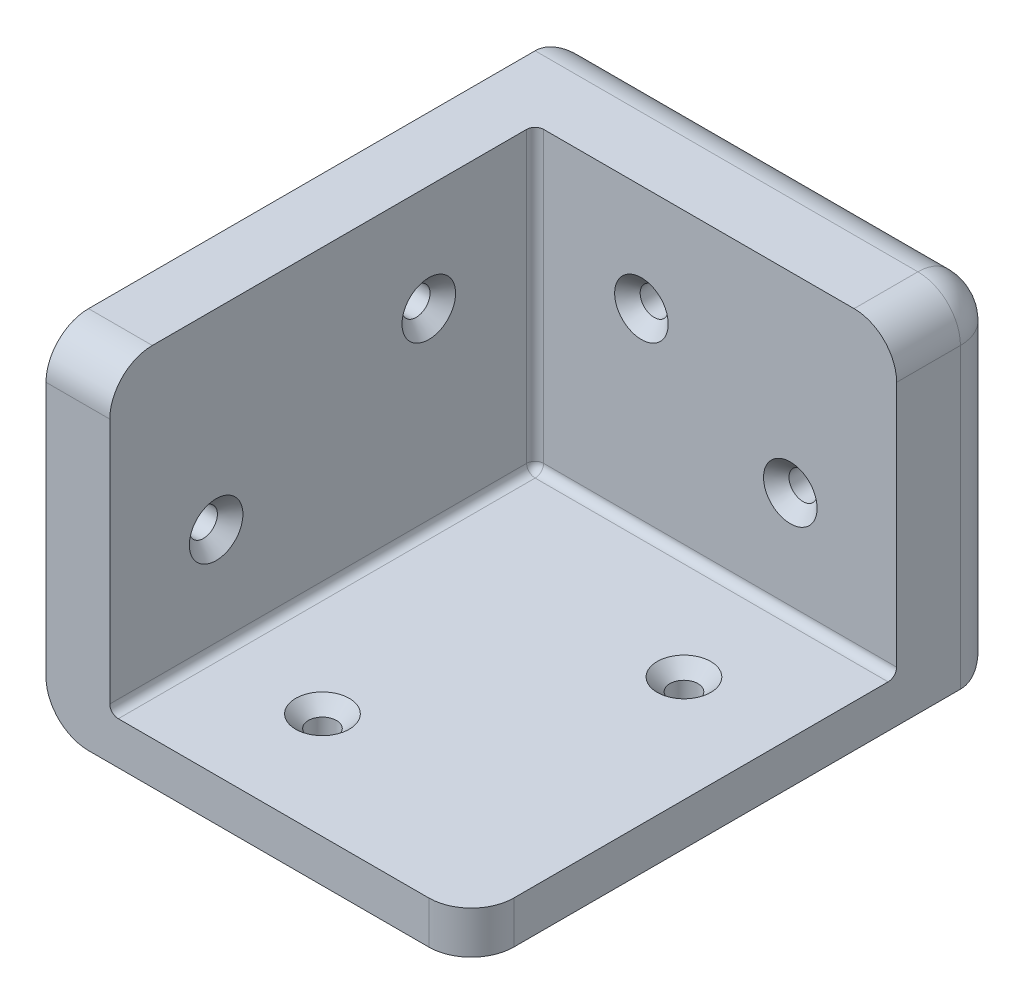
ISO-10303-21;
HEADER;
FILE_DESCRIPTION(('STEP AP214'),'2;1');
FILE_NAME('part.step','',(''),(''),'','','');
FILE_SCHEMA(('AUTOMOTIVE_DESIGN { 1 0 10303 214 1 1 1 1 }'));
ENDSEC;
DATA;
#1=APPLICATION_CONTEXT('core data for automotive mechanical design processes');
#2=APPLICATION_PROTOCOL_DEFINITION('international standard','automotive_design',2000,#1);
#3=PRODUCT_CONTEXT('',#1,'mechanical');
#4=PRODUCT('Part','Part','',(#3));
#5=PRODUCT_RELATED_PRODUCT_CATEGORY('part','',(#4));
#6=PRODUCT_DEFINITION_FORMATION('','',#4);
#7=PRODUCT_DEFINITION_CONTEXT('part definition',#1,'design');
#8=PRODUCT_DEFINITION('design','',#6,#7);
#9=PRODUCT_DEFINITION_SHAPE('','',#8);
#10=(LENGTH_UNIT() NAMED_UNIT(*) SI_UNIT(.MILLI.,.METRE.));
#11=(NAMED_UNIT(*) PLANE_ANGLE_UNIT() SI_UNIT($,.RADIAN.));
#12=(NAMED_UNIT(*) SI_UNIT($,.STERADIAN.) SOLID_ANGLE_UNIT());
#13=UNCERTAINTY_MEASURE_WITH_UNIT(LENGTH_MEASURE(1.E-05),#10,'distance_accuracy_value','');
#14=(GEOMETRIC_REPRESENTATION_CONTEXT(3) GLOBAL_UNCERTAINTY_ASSIGNED_CONTEXT((#13)) GLOBAL_UNIT_ASSIGNED_CONTEXT((#10,
#11,#12)) REPRESENTATION_CONTEXT('',''));
#15=CARTESIAN_POINT('',(0.,0.,0.));
#16=DIRECTION('',(0.,0.,1.));
#17=DIRECTION('',(1.,0.,0.));
#18=AXIS2_PLACEMENT_3D('',#15,#16,#17);
#19=CARTESIAN_POINT('',(-50.,40.,125.));
#20=DIRECTION('',(1.,0.,0.));
#21=DIRECTION('',(0.,1.,0.));
#22=AXIS2_PLACEMENT_3D('',#19,#20,#21);
#23=PLANE('',#22);
#24=CARTESIAN_POINT('',(-50.,-5.00000000000002,100.));
#25=DIRECTION('',(1.,0.,0.));
#26=DIRECTION('',(0.,1.,0.));
#27=AXIS2_PLACEMENT_3D('',#24,#25,#26);
#28=CIRCLE('',#27,3.29999999999999);
#29=CARTESIAN_POINT('',(-50.,-1.70000000000002,100.));
#30=VERTEX_POINT('',#29);
#31=EDGE_CURVE('E183',#30,#30,#28,.T.);
#32=ORIENTED_EDGE('',*,*,#31,.T.);
#33=EDGE_LOOP('',(#32));
#34=FACE_BOUND('',#33,.T.);
#35=CARTESIAN_POINT('',(-50.,15.,50.));
#36=DIRECTION('',(1.,0.,0.));
#37=DIRECTION('',(0.,1.,0.));
#38=AXIS2_PLACEMENT_3D('',#35,#36,#37);
#39=CIRCLE('',#38,3.29999999999999);
#40=CARTESIAN_POINT('',(-50.,18.3,50.));
#41=VERTEX_POINT('',#40);
#42=EDGE_CURVE('E323',#41,#41,#39,.T.);
#43=ORIENTED_EDGE('',*,*,#42,.T.);
#44=EDGE_LOOP('',(#43));
#45=FACE_BOUND('',#44,.T.);
#46=DIRECTION('',(0.,-1.,0.));
#47=VECTOR('',#46,1.);
#48=CARTESIAN_POINT('',(-50.,-40.,9.99999999999999));
#49=LINE('',#48,#47);
#50=CARTESIAN_POINT('',(-50.,40.,9.99999999999999));
#51=VERTEX_POINT('',#50);
#52=CARTESIAN_POINT('',(-50.,-30.,9.99999999999999));
#53=VERTEX_POINT('',#52);
#54=EDGE_CURVE('E193',#51,#53,#49,.T.);
#55=ORIENTED_EDGE('',*,*,#54,.T.);
#56=DIRECTION('',(0.,0.,-1.));
#57=VECTOR('',#56,1.);
#58=CARTESIAN_POINT('',(-50.,-30.,125.));
#59=LINE('',#58,#57);
#60=CARTESIAN_POINT('',(-50.,-30.,125.));
#61=VERTEX_POINT('',#60);
#62=EDGE_CURVE('E192',#53,#61,#59,.F.);
#63=ORIENTED_EDGE('',*,*,#62,.T.);
#64=DIRECTION('',(0.,-1.,0.));
#65=VECTOR('',#64,1.);
#66=CARTESIAN_POINT('',(-50.,40.,125.));
#67=LINE('',#66,#65);
#68=CARTESIAN_POINT('',(-50.,30.,125.));
#69=VERTEX_POINT('',#68);
#70=EDGE_CURVE('E290',#69,#61,#67,.T.);
#71=ORIENTED_EDGE('',*,*,#70,.F.);
#72=CARTESIAN_POINT('',(-50.,30.,115.));
#73=DIRECTION('',(1.,0.,0.));
#74=DIRECTION('',(0.,1.,0.));
#75=AXIS2_PLACEMENT_3D('',#72,#73,#74);
#76=CIRCLE('',#75,10.);
#77=CARTESIAN_POINT('',(-50.,40.,115.));
#78=VERTEX_POINT('',#77);
#79=EDGE_CURVE('E190',#69,#78,#76,.F.);
#80=ORIENTED_EDGE('',*,*,#79,.T.);
#81=DIRECTION('',(0.,0.,-1.));
#82=VECTOR('',#81,1.);
#83=CARTESIAN_POINT('',(-50.,40.,125.));
#84=LINE('',#83,#82);
#85=EDGE_CURVE('E171',#78,#51,#84,.T.);
#86=ORIENTED_EDGE('',*,*,#85,.T.);
#87=EDGE_LOOP('',(#55,#63,#71,#80,#86));
#88=FACE_BOUND('',#87,.T.);
#89=ADVANCED_FACE('F41',(#34,#45,#88),#23,.F.);
#90=CARTESIAN_POINT('',(50.,-40.,125.));
#91=DIRECTION('',(0.,1.,0.));
#92=DIRECTION('',(-1.,0.,0.));
#93=AXIS2_PLACEMENT_3D('',#90,#91,#92);
#94=PLANE('',#93);
#95=CARTESIAN_POINT('',(-10.,-40.,100.));
#96=DIRECTION('',(0.,1.,0.));
#97=DIRECTION('',(-1.,0.,0.));
#98=AXIS2_PLACEMENT_3D('',#95,#96,#97);
#99=CIRCLE('',#98,3.29999999999999);
#100=CARTESIAN_POINT('',(-13.3,-40.,100.));
#101=VERTEX_POINT('',#100);
#102=EDGE_CURVE('E317',#101,#101,#99,.T.);
#103=ORIENTED_EDGE('',*,*,#102,.T.);
#104=EDGE_LOOP('',(#103));
#105=FACE_BOUND('',#104,.T.);
#106=CARTESIAN_POINT('',(25.,-40.,50.));
#107=DIRECTION('',(0.,1.,0.));
#108=DIRECTION('',(-1.,0.,0.));
#109=AXIS2_PLACEMENT_3D('',#106,#107,#108);
#110=CIRCLE('',#109,3.29999999999999);
#111=CARTESIAN_POINT('',(21.7,-40.,50.));
#112=VERTEX_POINT('',#111);
#113=EDGE_CURVE('E314',#112,#112,#110,.T.);
#114=ORIENTED_EDGE('',*,*,#113,.T.);
#115=EDGE_LOOP('',(#114));
#116=FACE_BOUND('',#115,.T.);
#117=DIRECTION('',(1.,0.,0.));
#118=VECTOR('',#117,1.);
#119=CARTESIAN_POINT('',(50.,-40.,125.));
#120=LINE('',#119,#118);
#121=CARTESIAN_POINT('',(-40.,-40.,125.));
#122=VERTEX_POINT('',#121);
#123=CARTESIAN_POINT('',(40.,-40.,125.));
#124=VERTEX_POINT('',#123);
#125=EDGE_CURVE('E295',#122,#124,#120,.T.);
#126=ORIENTED_EDGE('',*,*,#125,.F.);
#127=DIRECTION('',(0.,0.,-1.));
#128=VECTOR('',#127,1.);
#129=CARTESIAN_POINT('',(-40.,-40.,125.));
#130=LINE('',#129,#128);
#131=CARTESIAN_POINT('',(-40.,-40.,9.99999999999999));
#132=VERTEX_POINT('',#131);
#133=EDGE_CURVE('E185',#122,#132,#130,.T.);
#134=ORIENTED_EDGE('',*,*,#133,.T.);
#135=DIRECTION('',(1.,0.,0.));
#136=VECTOR('',#135,1.);
#137=CARTESIAN_POINT('',(50.,-40.,9.99999999999999));
#138=LINE('',#137,#136);
#139=CARTESIAN_POINT('',(50.,-40.,9.99999999999999));
#140=VERTEX_POINT('',#139);
#141=EDGE_CURVE('E175',#132,#140,#138,.T.);
#142=ORIENTED_EDGE('',*,*,#141,.T.);
#143=DIRECTION('',(0.,0.,-1.));
#144=VECTOR('',#143,1.);
#145=CARTESIAN_POINT('',(50.,-40.,125.));
#146=LINE('',#145,#144);
#147=CARTESIAN_POINT('',(50.,-40.,115.));
#148=VERTEX_POINT('',#147);
#149=EDGE_CURVE('E156',#148,#140,#146,.T.);
#150=ORIENTED_EDGE('',*,*,#149,.F.);
#151=CARTESIAN_POINT('',(40.,-40.,115.));
#152=DIRECTION('',(0.,1.,0.));
#153=DIRECTION('',(-1.,0.,0.));
#154=AXIS2_PLACEMENT_3D('',#151,#152,#153);
#155=CIRCLE('',#154,10.);
#156=EDGE_CURVE('E168',#148,#124,#155,.F.);
#157=ORIENTED_EDGE('',*,*,#156,.T.);
#158=EDGE_LOOP('',(#126,#134,#142,#150,#157));
#159=FACE_BOUND('',#158,.T.);
#160=ADVANCED_FACE('F166',(#105,#116,#159),#94,.F.);
#161=CARTESIAN_POINT('',(50.,40.,125.));
#162=DIRECTION('',(-1.,0.,0.));
#163=DIRECTION('',(0.,-1.,0.));
#164=AXIS2_PLACEMENT_3D('',#161,#162,#163);
#165=PLANE('',#164);
#166=ORIENTED_EDGE('',*,*,#149,.T.);
#167=DIRECTION('',(0.,1.,0.));
#168=VECTOR('',#167,1.);
#169=CARTESIAN_POINT('',(50.,40.,9.99999999999999));
#170=LINE('',#169,#168);
#171=CARTESIAN_POINT('',(50.,30.,9.99999999999999));
#172=VERTEX_POINT('',#171);
#173=EDGE_CURVE('E217',#140,#172,#170,.T.);
#174=ORIENTED_EDGE('',*,*,#173,.T.);
#175=DIRECTION('',(0.,0.,-1.));
#176=VECTOR('',#175,1.);
#177=CARTESIAN_POINT('',(50.,30.,125.));
#178=LINE('',#177,#176);
#179=CARTESIAN_POINT('',(50.,30.,25.));
#180=VERTEX_POINT('',#179);
#181=EDGE_CURVE('E163',#172,#180,#178,.F.);
#182=ORIENTED_EDGE('',*,*,#181,.T.);
#183=DIRECTION('',(0.,1.,0.));
#184=VECTOR('',#183,1.);
#185=CARTESIAN_POINT('',(50.,40.,25.));
#186=LINE('',#185,#184);
#187=CARTESIAN_POINT('',(50.,-28.,25.));
#188=VERTEX_POINT('',#187);
#189=EDGE_CURVE('E285',#188,#180,#186,.T.);
#190=ORIENTED_EDGE('',*,*,#189,.F.);
#191=CARTESIAN_POINT('',(50.,-28.,27.));
#192=DIRECTION('',(-1.,0.,0.));
#193=DIRECTION('',(0.,-1.,0.));
#194=AXIS2_PLACEMENT_3D('',#191,#192,#193);
#195=CIRCLE('',#194,2.);
#196=CARTESIAN_POINT('',(50.,-30.,27.));
#197=VERTEX_POINT('',#196);
#198=EDGE_CURVE('E265',#188,#197,#195,.T.);
#199=ORIENTED_EDGE('',*,*,#198,.T.);
#200=DIRECTION('',(0.,0.,1.));
#201=VECTOR('',#200,1.);
#202=CARTESIAN_POINT('',(50.,-30.,-110.113577727726));
#203=LINE('',#202,#201);
#204=CARTESIAN_POINT('',(50.,-30.,115.));
#205=VERTEX_POINT('',#204);
#206=EDGE_CURVE('E157',#197,#205,#203,.T.);
#207=ORIENTED_EDGE('',*,*,#206,.T.);
#208=DIRECTION('',(0.,1.,0.));
#209=VECTOR('',#208,1.);
#210=CARTESIAN_POINT('',(50.,40.,115.));
#211=LINE('',#210,#209);
#212=EDGE_CURVE('E153',#205,#148,#211,.F.);
#213=ORIENTED_EDGE('',*,*,#212,.T.);
#214=EDGE_LOOP('',(#166,#174,#182,#190,#199,#207,#213));
#215=FACE_BOUND('',#214,.T.);
#216=ADVANCED_FACE('F154',(#215),#165,.F.);
#217=CARTESIAN_POINT('',(50.,40.,125.));
#218=DIRECTION('',(0.,-1.,0.));
#219=DIRECTION('',(1.,0.,0.));
#220=AXIS2_PLACEMENT_3D('',#217,#218,#219);
#221=PLANE('',#220);
#222=DIRECTION('',(0.,0.,-1.));
#223=VECTOR('',#222,1.);
#224=CARTESIAN_POINT('',(40.,40.,125.));
#225=LINE('',#224,#223);
#226=CARTESIAN_POINT('',(40.,40.,25.));
#227=VERTEX_POINT('',#226);
#228=CARTESIAN_POINT('',(40.,40.,9.99999999999999));
#229=VERTEX_POINT('',#228);
#230=EDGE_CURVE('E204',#227,#229,#225,.T.);
#231=ORIENTED_EDGE('',*,*,#230,.T.);
#232=DIRECTION('',(-1.,0.,0.));
#233=VECTOR('',#232,1.);
#234=CARTESIAN_POINT('',(-50.,40.,9.99999999999999));
#235=LINE('',#234,#233);
#236=EDGE_CURVE('E206',#229,#51,#235,.T.);
#237=ORIENTED_EDGE('',*,*,#236,.T.);
#238=ORIENTED_EDGE('',*,*,#85,.F.);
#239=DIRECTION('',(-1.,0.,0.));
#240=VECTOR('',#239,1.);
#241=CARTESIAN_POINT('',(50.,40.,115.));
#242=LINE('',#241,#240);
#243=CARTESIAN_POINT('',(-35.,40.,115.));
#244=VERTEX_POINT('',#243);
#245=EDGE_CURVE('E203',#78,#244,#242,.F.);
#246=ORIENTED_EDGE('',*,*,#245,.T.);
#247=DIRECTION('',(0.,0.,1.));
#248=VECTOR('',#247,1.);
#249=CARTESIAN_POINT('',(-35.,40.,-110.113577727726));
#250=LINE('',#249,#248);
#251=CARTESIAN_POINT('',(-35.,40.,27.));
#252=VERTEX_POINT('',#251);
#253=EDGE_CURVE('E294',#252,#244,#250,.T.);
#254=ORIENTED_EDGE('',*,*,#253,.F.);
#255=CARTESIAN_POINT('',(-33.,40.,27.));
#256=DIRECTION('',(0.,-1.,0.));
#257=DIRECTION('',(1.,0.,0.));
#258=AXIS2_PLACEMENT_3D('',#255,#256,#257);
#259=CIRCLE('',#258,2.);
#260=CARTESIAN_POINT('',(-33.,40.,25.));
#261=VERTEX_POINT('',#260);
#262=EDGE_CURVE('E49',#252,#261,#259,.T.);
#263=ORIENTED_EDGE('',*,*,#262,.T.);
#264=DIRECTION('',(-1.,0.,0.));
#265=VECTOR('',#264,1.);
#266=CARTESIAN_POINT('',(50.,40.,25.));
#267=LINE('',#266,#265);
#268=EDGE_CURVE('E299',#227,#261,#267,.T.);
#269=ORIENTED_EDGE('',*,*,#268,.F.);
#270=EDGE_LOOP('',(#231,#237,#238,#246,#254,#263,#269));
#271=FACE_BOUND('',#270,.T.);
#272=ADVANCED_FACE('F392',(#271),#221,.F.);
#273=CARTESIAN_POINT('',(0.,0.,125.));
#274=DIRECTION('',(0.,0.,-1.));
#275=DIRECTION('',(-1.,0.,0.));
#276=AXIS2_PLACEMENT_3D('',#273,#274,#275);
#277=PLANE('',#276);
#278=ORIENTED_EDGE('',*,*,#70,.T.);
#279=CARTESIAN_POINT('',(-40.,-30.,125.));
#280=DIRECTION('',(0.,0.,-1.));
#281=DIRECTION('',(-1.,0.,0.));
#282=AXIS2_PLACEMENT_3D('',#279,#280,#281);
#283=CIRCLE('',#282,10.);
#284=EDGE_CURVE('E200',#61,#122,#283,.F.);
#285=ORIENTED_EDGE('',*,*,#284,.T.);
#286=ORIENTED_EDGE('',*,*,#125,.T.);
#287=DIRECTION('',(0.,1.,0.));
#288=VECTOR('',#287,1.);
#289=CARTESIAN_POINT('',(40.,0.,125.));
#290=LINE('',#289,#288);
#291=CARTESIAN_POINT('',(40.,-30.,125.));
#292=VERTEX_POINT('',#291);
#293=EDGE_CURVE('E176',#124,#292,#290,.T.);
#294=ORIENTED_EDGE('',*,*,#293,.T.);
#295=DIRECTION('',(1.,0.,0.));
#296=VECTOR('',#295,1.);
#297=CARTESIAN_POINT('',(50.,-30.,125.));
#298=LINE('',#297,#296);
#299=CARTESIAN_POINT('',(-33.,-30.,125.));
#300=VERTEX_POINT('',#299);
#301=EDGE_CURVE('E355',#300,#292,#298,.T.);
#302=ORIENTED_EDGE('',*,*,#301,.F.);
#303=CARTESIAN_POINT('',(-33.,-28.,125.));
#304=DIRECTION('',(0.,0.,-1.));
#305=DIRECTION('',(-1.,0.,0.));
#306=AXIS2_PLACEMENT_3D('',#303,#304,#305);
#307=CIRCLE('',#306,2.);
#308=CARTESIAN_POINT('',(-35.,-28.,125.));
#309=VERTEX_POINT('',#308);
#310=EDGE_CURVE('E12',#300,#309,#307,.T.);
#311=ORIENTED_EDGE('',*,*,#310,.T.);
#312=DIRECTION('',(0.,-1.,0.));
#313=VECTOR('',#312,1.);
#314=CARTESIAN_POINT('',(-35.,40.,125.));
#315=LINE('',#314,#313);
#316=CARTESIAN_POINT('',(-35.,30.,125.));
#317=VERTEX_POINT('',#316);
#318=EDGE_CURVE('E307',#317,#309,#315,.T.);
#319=ORIENTED_EDGE('',*,*,#318,.F.);
#320=DIRECTION('',(-1.,0.,0.));
#321=VECTOR('',#320,1.);
#322=CARTESIAN_POINT('',(0.,30.,125.));
#323=LINE('',#322,#321);
#324=EDGE_CURVE('E198',#317,#69,#323,.T.);
#325=ORIENTED_EDGE('',*,*,#324,.T.);
#326=EDGE_LOOP('',(#278,#285,#286,#294,#302,#311,#319,#325));
#327=FACE_BOUND('',#326,.T.);
#328=ADVANCED_FACE('F356',(#327),#277,.F.);
#329=CARTESIAN_POINT('',(0.,0.,0.));
#330=DIRECTION('',(0.,0.,-1.));
#331=DIRECTION('',(-1.,0.,0.));
#332=AXIS2_PLACEMENT_3D('',#329,#330,#331);
#333=PLANE('',#332);
#334=DIRECTION('',(0.,-1.,0.));
#335=VECTOR('',#334,1.);
#336=CARTESIAN_POINT('',(-40.,40.,0.));
#337=LINE('',#336,#335);
#338=CARTESIAN_POINT('',(-40.,-30.,0.));
#339=VERTEX_POINT('',#338);
#340=CARTESIAN_POINT('',(-40.,30.,0.));
#341=VERTEX_POINT('',#340);
#342=EDGE_CURVE('E215',#339,#341,#337,.F.);
#343=ORIENTED_EDGE('',*,*,#342,.T.);
#344=DIRECTION('',(-1.,0.,0.));
#345=VECTOR('',#344,1.);
#346=CARTESIAN_POINT('',(50.,30.,0.));
#347=LINE('',#346,#345);
#348=CARTESIAN_POINT('',(40.,30.,0.));
#349=VERTEX_POINT('',#348);
#350=EDGE_CURVE('E164',#341,#349,#347,.F.);
#351=ORIENTED_EDGE('',*,*,#350,.T.);
#352=DIRECTION('',(0.,1.,0.));
#353=VECTOR('',#352,1.);
#354=CARTESIAN_POINT('',(40.,-40.,0.));
#355=LINE('',#354,#353);
#356=CARTESIAN_POINT('',(40.,-30.,0.));
#357=VERTEX_POINT('',#356);
#358=EDGE_CURVE('E208',#349,#357,#355,.F.);
#359=ORIENTED_EDGE('',*,*,#358,.T.);
#360=DIRECTION('',(1.,0.,0.));
#361=VECTOR('',#360,1.);
#362=CARTESIAN_POINT('',(-50.,-30.,0.));
#363=LINE('',#362,#361);
#364=EDGE_CURVE('E209',#357,#339,#363,.F.);
#365=ORIENTED_EDGE('',*,*,#364,.T.);
#366=EDGE_LOOP('',(#343,#351,#359,#365));
#367=FACE_BOUND('',#366,.T.);
#368=CARTESIAN_POINT('',(25.,-5.,0.));
#369=DIRECTION('',(0.,0.,-1.));
#370=DIRECTION('',(-1.,0.,0.));
#371=AXIS2_PLACEMENT_3D('',#368,#369,#370);
#372=CIRCLE('',#371,3.29999999999999);
#373=CARTESIAN_POINT('',(21.7,-5.,0.));
#374=VERTEX_POINT('',#373);
#375=EDGE_CURVE('E310',#374,#374,#372,.T.);
#376=ORIENTED_EDGE('',*,*,#375,.F.);
#377=EDGE_LOOP('',(#376));
#378=FACE_BOUND('',#377,.T.);
#379=CARTESIAN_POINT('',(-10.,15.,0.));
#380=DIRECTION('',(0.,0.,-1.));
#381=DIRECTION('',(-1.,0.,0.));
#382=AXIS2_PLACEMENT_3D('',#379,#380,#381);
#383=CIRCLE('',#382,3.29999999999999);
#384=CARTESIAN_POINT('',(-13.3,15.,0.));
#385=VERTEX_POINT('',#384);
#386=EDGE_CURVE('E305',#385,#385,#383,.T.);
#387=ORIENTED_EDGE('',*,*,#386,.F.);
#388=EDGE_LOOP('',(#387));
#389=FACE_BOUND('',#388,.T.);
#390=ADVANCED_FACE('F666',(#367,#378,#389),#333,.T.);
#391=CARTESIAN_POINT('',(0.,0.,25.));
#392=DIRECTION('',(0.,0.,-1.));
#393=DIRECTION('',(-1.,0.,0.));
#394=AXIS2_PLACEMENT_3D('',#391,#392,#393);
#395=PLANE('',#394);
#396=CARTESIAN_POINT('',(25.,-5.,25.));
#397=DIRECTION('',(0.,0.,1.));
#398=DIRECTION('',(1.,0.,0.));
#399=AXIS2_PLACEMENT_3D('',#396,#397,#398);
#400=CIRCLE('',#399,6.3);
#401=CARTESIAN_POINT('',(31.3,-5.,25.));
#402=VERTEX_POINT('',#401);
#403=EDGE_CURVE('E320',#402,#402,#400,.T.);
#404=ORIENTED_EDGE('',*,*,#403,.F.);
#405=EDGE_LOOP('',(#404));
#406=FACE_BOUND('',#405,.T.);
#407=CARTESIAN_POINT('',(-10.,15.,25.));
#408=DIRECTION('',(0.,0.,1.));
#409=DIRECTION('',(1.,0.,0.));
#410=AXIS2_PLACEMENT_3D('',#407,#408,#409);
#411=CIRCLE('',#410,6.3);
#412=CARTESIAN_POINT('',(-3.70000000000002,15.,25.));
#413=VERTEX_POINT('',#412);
#414=EDGE_CURVE('E315',#413,#413,#411,.T.);
#415=ORIENTED_EDGE('',*,*,#414,.F.);
#416=EDGE_LOOP('',(#415));
#417=FACE_BOUND('',#416,.T.);
#418=DIRECTION('',(0.,-1.,0.));
#419=VECTOR('',#418,1.);
#420=CARTESIAN_POINT('',(-33.,-30.,25.));
#421=LINE('',#420,#419);
#422=CARTESIAN_POINT('',(-33.,-28.,25.));
#423=VERTEX_POINT('',#422);
#424=EDGE_CURVE('E228',#261,#423,#421,.T.);
#425=ORIENTED_EDGE('',*,*,#424,.T.);
#426=DIRECTION('',(1.,0.,0.));
#427=VECTOR('',#426,1.);
#428=CARTESIAN_POINT('',(50.,-28.,25.));
#429=LINE('',#428,#427);
#430=EDGE_CURVE('E252',#423,#188,#429,.T.);
#431=ORIENTED_EDGE('',*,*,#430,.T.);
#432=ORIENTED_EDGE('',*,*,#189,.T.);
#433=CARTESIAN_POINT('',(40.,30.,25.));
#434=DIRECTION('',(0.,0.,-1.));
#435=DIRECTION('',(-1.,0.,0.));
#436=AXIS2_PLACEMENT_3D('',#433,#434,#435);
#437=CIRCLE('',#436,10.);
#438=EDGE_CURVE('E219',#180,#227,#437,.F.);
#439=ORIENTED_EDGE('',*,*,#438,.T.);
#440=ORIENTED_EDGE('',*,*,#268,.T.);
#441=EDGE_LOOP('',(#425,#431,#432,#439,#440));
#442=FACE_BOUND('',#441,.T.);
#443=ADVANCED_FACE('F282',(#406,#417,#442),#395,.F.);
#444=CARTESIAN_POINT('',(-35.,40.,-110.113577727726));
#445=DIRECTION('',(-1.,0.,0.));
#446=DIRECTION('',(0.,-1.,0.));
#447=AXIS2_PLACEMENT_3D('',#444,#445,#446);
#448=PLANE('',#447);
#449=CARTESIAN_POINT('',(-35.,-5.00000000000002,100.));
#450=DIRECTION('',(1.,0.,0.));
#451=DIRECTION('',(0.,0.,-1.));
#452=AXIS2_PLACEMENT_3D('',#449,#450,#451);
#453=CIRCLE('',#452,6.3);
#454=CARTESIAN_POINT('',(-35.,-5.00000000000002,93.7));
#455=VERTEX_POINT('',#454);
#456=EDGE_CURVE('E246',#455,#455,#453,.T.);
#457=ORIENTED_EDGE('',*,*,#456,.F.);
#458=EDGE_LOOP('',(#457));
#459=FACE_BOUND('',#458,.T.);
#460=CARTESIAN_POINT('',(-35.,15.,50.));
#461=DIRECTION('',(1.,0.,0.));
#462=DIRECTION('',(0.,0.,-1.));
#463=AXIS2_PLACEMENT_3D('',#460,#461,#462);
#464=CIRCLE('',#463,6.3);
#465=CARTESIAN_POINT('',(-35.,15.,43.7));
#466=VERTEX_POINT('',#465);
#467=EDGE_CURVE('E335',#466,#466,#464,.T.);
#468=ORIENTED_EDGE('',*,*,#467,.F.);
#469=EDGE_LOOP('',(#468));
#470=FACE_BOUND('',#469,.T.);
#471=DIRECTION('',(0.,0.,1.));
#472=VECTOR('',#471,1.);
#473=CARTESIAN_POINT('',(-35.,-28.,25.));
#474=LINE('',#473,#472);
#475=CARTESIAN_POINT('',(-35.,-28.,27.));
#476=VERTEX_POINT('',#475);
#477=EDGE_CURVE('E59',#309,#476,#474,.F.);
#478=ORIENTED_EDGE('',*,*,#477,.T.);
#479=DIRECTION('',(0.,-1.,0.));
#480=VECTOR('',#479,1.);
#481=CARTESIAN_POINT('',(-35.,40.,27.));
#482=LINE('',#481,#480);
#483=EDGE_CURVE('E257',#476,#252,#482,.F.);
#484=ORIENTED_EDGE('',*,*,#483,.T.);
#485=ORIENTED_EDGE('',*,*,#253,.T.);
#486=CARTESIAN_POINT('',(-35.,30.,115.));
#487=DIRECTION('',(-1.,0.,0.));
#488=DIRECTION('',(0.,-1.,0.));
#489=AXIS2_PLACEMENT_3D('',#486,#487,#488);
#490=CIRCLE('',#489,10.);
#491=EDGE_CURVE('E225',#244,#317,#490,.F.);
#492=ORIENTED_EDGE('',*,*,#491,.T.);
#493=ORIENTED_EDGE('',*,*,#318,.T.);
#494=EDGE_LOOP('',(#478,#484,#485,#492,#493));
#495=FACE_BOUND('',#494,.T.);
#496=ADVANCED_FACE('F351',(#459,#470,#495),#448,.F.);
#497=CARTESIAN_POINT('',(50.,-30.,-110.113577727726));
#498=DIRECTION('',(0.,-1.,0.));
#499=DIRECTION('',(1.,0.,0.));
#500=AXIS2_PLACEMENT_3D('',#497,#498,#499);
#501=PLANE('',#500);
#502=CARTESIAN_POINT('',(-10.,-30.,100.));
#503=DIRECTION('',(0.,1.,0.));
#504=DIRECTION('',(0.,0.,1.));
#505=AXIS2_PLACEMENT_3D('',#502,#503,#504);
#506=CIRCLE('',#505,6.3);
#507=CARTESIAN_POINT('',(-10.,-30.,106.3));
#508=VERTEX_POINT('',#507);
#509=EDGE_CURVE('E324',#508,#508,#506,.T.);
#510=ORIENTED_EDGE('',*,*,#509,.F.);
#511=EDGE_LOOP('',(#510));
#512=FACE_BOUND('',#511,.T.);
#513=CARTESIAN_POINT('',(25.,-30.,50.));
#514=DIRECTION('',(0.,1.,0.));
#515=DIRECTION('',(0.,0.,1.));
#516=AXIS2_PLACEMENT_3D('',#513,#514,#515);
#517=CIRCLE('',#516,6.3);
#518=CARTESIAN_POINT('',(25.,-30.,56.3));
#519=VERTEX_POINT('',#518);
#520=EDGE_CURVE('E321',#519,#519,#517,.T.);
#521=ORIENTED_EDGE('',*,*,#520,.F.);
#522=EDGE_LOOP('',(#521));
#523=FACE_BOUND('',#522,.T.);
#524=ORIENTED_EDGE('',*,*,#206,.F.);
#525=DIRECTION('',(1.,0.,0.));
#526=VECTOR('',#525,1.);
#527=CARTESIAN_POINT('',(-35.,-30.,27.));
#528=LINE('',#527,#526);
#529=CARTESIAN_POINT('',(-33.,-30.,27.));
#530=VERTEX_POINT('',#529);
#531=EDGE_CURVE('E260',#197,#530,#528,.F.);
#532=ORIENTED_EDGE('',*,*,#531,.T.);
#533=DIRECTION('',(0.,0.,1.));
#534=VECTOR('',#533,1.);
#535=CARTESIAN_POINT('',(-33.,-30.,125.));
#536=LINE('',#535,#534);
#537=EDGE_CURVE('E254',#530,#300,#536,.T.);
#538=ORIENTED_EDGE('',*,*,#537,.T.);
#539=ORIENTED_EDGE('',*,*,#301,.T.);
#540=CARTESIAN_POINT('',(40.,-30.,115.));
#541=DIRECTION('',(0.,-1.,0.));
#542=DIRECTION('',(1.,0.,0.));
#543=AXIS2_PLACEMENT_3D('',#540,#541,#542);
#544=CIRCLE('',#543,10.);
#545=EDGE_CURVE('E221',#292,#205,#544,.F.);
#546=ORIENTED_EDGE('',*,*,#545,.T.);
#547=EDGE_LOOP('',(#524,#532,#538,#539,#546));
#548=FACE_BOUND('',#547,.T.);
#549=ADVANCED_FACE('F360',(#512,#523,#548),#501,.F.);
#550=CARTESIAN_POINT('',(-10.,15.,25.));
#551=DIRECTION('',(0.,0.,1.));
#552=DIRECTION('',(1.,0.,0.));
#553=AXIS2_PLACEMENT_3D('',#550,#551,#552);
#554=CYLINDRICAL_SURFACE('',#553,3.29999999999999);
#555=ORIENTED_EDGE('',*,*,#386,.T.);
#556=EDGE_LOOP('',(#555));
#557=FACE_BOUND('',#556,.T.);
#558=CARTESIAN_POINT('',(-10.,15.,22.));
#559=DIRECTION('',(0.,0.,1.));
#560=DIRECTION('',(1.,0.,0.));
#561=AXIS2_PLACEMENT_3D('',#558,#559,#560);
#562=CIRCLE('',#561,3.3);
#563=CARTESIAN_POINT('',(-6.70000000000002,15.,22.));
#564=VERTEX_POINT('',#563);
#565=EDGE_CURVE('E306',#564,#564,#562,.T.);
#566=ORIENTED_EDGE('',*,*,#565,.T.);
#567=EDGE_LOOP('',(#566));
#568=FACE_BOUND('',#567,.T.);
#569=ADVANCED_FACE('F635',(#557,#568),#554,.F.);
#570=CARTESIAN_POINT('',(-10.,15.,25.));
#571=DIRECTION('',(0.,0.,1.));
#572=DIRECTION('',(1.,0.,0.));
#573=AXIS2_PLACEMENT_3D('',#570,#571,#572);
#574=CONICAL_SURFACE('',#573,6.3,0.785398163397449);
#575=ORIENTED_EDGE('',*,*,#565,.F.);
#576=EDGE_LOOP('',(#575));
#577=FACE_BOUND('',#576,.T.);
#578=ORIENTED_EDGE('',*,*,#414,.T.);
#579=EDGE_LOOP('',(#578));
#580=FACE_BOUND('',#579,.T.);
#581=ADVANCED_FACE('F624',(#577,#580),#574,.F.);
#582=CARTESIAN_POINT('',(25.,-5.,25.));
#583=DIRECTION('',(0.,0.,1.));
#584=DIRECTION('',(1.,0.,0.));
#585=AXIS2_PLACEMENT_3D('',#582,#583,#584);
#586=CYLINDRICAL_SURFACE('',#585,3.29999999999999);
#587=ORIENTED_EDGE('',*,*,#375,.T.);
#588=EDGE_LOOP('',(#587));
#589=FACE_BOUND('',#588,.T.);
#590=CARTESIAN_POINT('',(25.,-5.,22.));
#591=DIRECTION('',(0.,0.,1.));
#592=DIRECTION('',(1.,0.,0.));
#593=AXIS2_PLACEMENT_3D('',#590,#591,#592);
#594=CIRCLE('',#593,3.29999999999999);
#595=CARTESIAN_POINT('',(28.3,-5.,22.));
#596=VERTEX_POINT('',#595);
#597=EDGE_CURVE('E311',#596,#596,#594,.T.);
#598=ORIENTED_EDGE('',*,*,#597,.T.);
#599=EDGE_LOOP('',(#598));
#600=FACE_BOUND('',#599,.T.);
#601=ADVANCED_FACE('F615',(#589,#600),#586,.F.);
#602=CARTESIAN_POINT('',(25.,-5.,25.));
#603=DIRECTION('',(0.,0.,1.));
#604=DIRECTION('',(1.,0.,0.));
#605=AXIS2_PLACEMENT_3D('',#602,#603,#604);
#606=CONICAL_SURFACE('',#605,6.3,0.785398163397449);
#607=ORIENTED_EDGE('',*,*,#597,.F.);
#608=EDGE_LOOP('',(#607));
#609=FACE_BOUND('',#608,.T.);
#610=ORIENTED_EDGE('',*,*,#403,.T.);
#611=EDGE_LOOP('',(#610));
#612=FACE_BOUND('',#611,.T.);
#613=ADVANCED_FACE('F603',(#609,#612),#606,.F.);
#614=CARTESIAN_POINT('',(25.,-30.,50.));
#615=DIRECTION('',(0.,1.,0.));
#616=DIRECTION('',(0.,0.,1.));
#617=AXIS2_PLACEMENT_3D('',#614,#615,#616);
#618=CYLINDRICAL_SURFACE('',#617,3.29999999999999);
#619=CARTESIAN_POINT('',(25.,-33.,50.));
#620=DIRECTION('',(0.,1.,0.));
#621=DIRECTION('',(0.,0.,1.));
#622=AXIS2_PLACEMENT_3D('',#619,#620,#621);
#623=CIRCLE('',#622,3.29999999999999);
#624=CARTESIAN_POINT('',(25.,-33.,53.3));
#625=VERTEX_POINT('',#624);
#626=EDGE_CURVE('E318',#625,#625,#623,.T.);
#627=ORIENTED_EDGE('',*,*,#626,.T.);
#628=EDGE_LOOP('',(#627));
#629=FACE_BOUND('',#628,.T.);
#630=ORIENTED_EDGE('',*,*,#113,.F.);
#631=EDGE_LOOP('',(#630));
#632=FACE_BOUND('',#631,.T.);
#633=ADVANCED_FACE('F592',(#629,#632),#618,.F.);
#634=CARTESIAN_POINT('',(25.,-30.,50.));
#635=DIRECTION('',(0.,1.,0.));
#636=DIRECTION('',(0.,0.,1.));
#637=AXIS2_PLACEMENT_3D('',#634,#635,#636);
#638=CONICAL_SURFACE('',#637,6.3,0.785398163397449);
#639=ORIENTED_EDGE('',*,*,#626,.F.);
#640=EDGE_LOOP('',(#639));
#641=FACE_BOUND('',#640,.T.);
#642=ORIENTED_EDGE('',*,*,#520,.T.);
#643=EDGE_LOOP('',(#642));
#644=FACE_BOUND('',#643,.T.);
#645=ADVANCED_FACE('F585',(#641,#644),#638,.F.);
#646=CARTESIAN_POINT('',(-10.,-30.,100.));
#647=DIRECTION('',(0.,1.,0.));
#648=DIRECTION('',(0.,0.,1.));
#649=AXIS2_PLACEMENT_3D('',#646,#647,#648);
#650=CYLINDRICAL_SURFACE('',#649,3.29999999999999);
#651=CARTESIAN_POINT('',(-10.,-33.,100.));
#652=DIRECTION('',(0.,1.,0.));
#653=DIRECTION('',(0.,0.,1.));
#654=AXIS2_PLACEMENT_3D('',#651,#652,#653);
#655=CIRCLE('',#654,3.3);
#656=CARTESIAN_POINT('',(-10.,-33.,103.3));
#657=VERTEX_POINT('',#656);
#658=EDGE_CURVE('E325',#657,#657,#655,.T.);
#659=ORIENTED_EDGE('',*,*,#658,.T.);
#660=EDGE_LOOP('',(#659));
#661=FACE_BOUND('',#660,.T.);
#662=ORIENTED_EDGE('',*,*,#102,.F.);
#663=EDGE_LOOP('',(#662));
#664=FACE_BOUND('',#663,.T.);
#665=ADVANCED_FACE('F575',(#661,#664),#650,.F.);
#666=CARTESIAN_POINT('',(-10.,-30.,100.));
#667=DIRECTION('',(0.,1.,0.));
#668=DIRECTION('',(0.,0.,1.));
#669=AXIS2_PLACEMENT_3D('',#666,#667,#668);
#670=CONICAL_SURFACE('',#669,6.3,0.785398163397449);
#671=ORIENTED_EDGE('',*,*,#658,.F.);
#672=EDGE_LOOP('',(#671));
#673=FACE_BOUND('',#672,.T.);
#674=ORIENTED_EDGE('',*,*,#509,.T.);
#675=EDGE_LOOP('',(#674));
#676=FACE_BOUND('',#675,.T.);
#677=ADVANCED_FACE('F561',(#673,#676),#670,.F.);
#678=CARTESIAN_POINT('',(-35.,15.,50.));
#679=DIRECTION('',(1.,0.,0.));
#680=DIRECTION('',(0.,0.,-1.));
#681=AXIS2_PLACEMENT_3D('',#678,#679,#680);
#682=CYLINDRICAL_SURFACE('',#681,3.29999999999999);
#683=CARTESIAN_POINT('',(-38.,15.,50.));
#684=DIRECTION('',(1.,0.,0.));
#685=DIRECTION('',(0.,0.,-1.));
#686=AXIS2_PLACEMENT_3D('',#683,#684,#685);
#687=CIRCLE('',#686,3.29999999999999);
#688=CARTESIAN_POINT('',(-38.,15.,46.7));
#689=VERTEX_POINT('',#688);
#690=EDGE_CURVE('E326',#689,#689,#687,.T.);
#691=ORIENTED_EDGE('',*,*,#690,.T.);
#692=EDGE_LOOP('',(#691));
#693=FACE_BOUND('',#692,.T.);
#694=ORIENTED_EDGE('',*,*,#42,.F.);
#695=EDGE_LOOP('',(#694));
#696=FACE_BOUND('',#695,.T.);
#697=ADVANCED_FACE('F553',(#693,#696),#682,.F.);
#698=CARTESIAN_POINT('',(-35.,15.,50.));
#699=DIRECTION('',(1.,0.,0.));
#700=DIRECTION('',(0.,0.,-1.));
#701=AXIS2_PLACEMENT_3D('',#698,#699,#700);
#702=CONICAL_SURFACE('',#701,6.3,0.785398163397449);
#703=ORIENTED_EDGE('',*,*,#690,.F.);
#704=EDGE_LOOP('',(#703));
#705=FACE_BOUND('',#704,.T.);
#706=ORIENTED_EDGE('',*,*,#467,.T.);
#707=EDGE_LOOP('',(#706));
#708=FACE_BOUND('',#707,.T.);
#709=ADVANCED_FACE('F544',(#705,#708),#702,.F.);
#710=CARTESIAN_POINT('',(-35.,-5.00000000000002,100.));
#711=DIRECTION('',(1.,0.,0.));
#712=DIRECTION('',(0.,0.,-1.));
#713=AXIS2_PLACEMENT_3D('',#710,#711,#712);
#714=CYLINDRICAL_SURFACE('',#713,3.29999999999999);
#715=CARTESIAN_POINT('',(-38.,-5.00000000000002,100.));
#716=DIRECTION('',(1.,0.,0.));
#717=DIRECTION('',(0.,0.,-1.));
#718=AXIS2_PLACEMENT_3D('',#715,#716,#717);
#719=CIRCLE('',#718,3.3);
#720=CARTESIAN_POINT('',(-38.,-5.00000000000002,96.7));
#721=VERTEX_POINT('',#720);
#722=EDGE_CURVE('E734',#721,#721,#719,.T.);
#723=ORIENTED_EDGE('',*,*,#722,.T.);
#724=EDGE_LOOP('',(#723));
#725=FACE_BOUND('',#724,.T.);
#726=ORIENTED_EDGE('',*,*,#31,.F.);
#727=EDGE_LOOP('',(#726));
#728=FACE_BOUND('',#727,.T.);
#729=ADVANCED_FACE('F532',(#725,#728),#714,.F.);
#730=CARTESIAN_POINT('',(-35.,-5.00000000000002,100.));
#731=DIRECTION('',(1.,0.,0.));
#732=DIRECTION('',(0.,0.,-1.));
#733=AXIS2_PLACEMENT_3D('',#730,#731,#732);
#734=CONICAL_SURFACE('',#733,6.3,0.785398163397449);
#735=ORIENTED_EDGE('',*,*,#722,.F.);
#736=EDGE_LOOP('',(#735));
#737=FACE_BOUND('',#736,.T.);
#738=ORIENTED_EDGE('',*,*,#456,.T.);
#739=EDGE_LOOP('',(#738));
#740=FACE_BOUND('',#739,.T.);
#741=ADVANCED_FACE('F439',(#737,#740),#734,.F.);
#742=CARTESIAN_POINT('',(40.,30.,125.));
#743=DIRECTION('',(0.,0.,-1.));
#744=DIRECTION('',(-1.,0.,0.));
#745=AXIS2_PLACEMENT_3D('',#742,#743,#744);
#746=CYLINDRICAL_SURFACE('',#745,10.);
#747=CARTESIAN_POINT('',(40.,30.,9.99999999999999));
#748=DIRECTION('',(0.,0.,-1.));
#749=DIRECTION('',(-1.,0.,0.));
#750=AXIS2_PLACEMENT_3D('',#747,#748,#749);
#751=CIRCLE('',#750,10.);
#752=EDGE_CURVE('E249',#229,#172,#751,.T.);
#753=ORIENTED_EDGE('',*,*,#752,.F.);
#754=ORIENTED_EDGE('',*,*,#230,.F.);
#755=ORIENTED_EDGE('',*,*,#438,.F.);
#756=ORIENTED_EDGE('',*,*,#181,.F.);
#757=EDGE_LOOP('',(#753,#754,#755,#756));
#758=FACE_BOUND('',#757,.T.);
#759=ADVANCED_FACE('F379',(#758),#746,.T.);
#760=CARTESIAN_POINT('',(40.,30.,10.));
#761=DIRECTION('',(1.,0.,0.));
#762=DIRECTION('',(0.,0.,-1.));
#763=AXIS2_PLACEMENT_3D('',#760,#761,#762);
#764=SPHERICAL_SURFACE('',#763,10.);
#765=CARTESIAN_POINT('',(40.,30.,10.));
#766=DIRECTION('',(1.,0.,0.));
#767=DIRECTION('',(0.,0.,-1.));
#768=AXIS2_PLACEMENT_3D('',#765,#766,#767);
#769=CIRCLE('',#768,10.);
#770=EDGE_CURVE('E243',#229,#349,#769,.F.);
#771=ORIENTED_EDGE('',*,*,#770,.F.);
#772=ORIENTED_EDGE('',*,*,#752,.T.);
#773=CARTESIAN_POINT('',(40.,30.,9.99999999999999));
#774=DIRECTION('',(0.,1.,0.));
#775=DIRECTION('',(-1.,0.,0.));
#776=AXIS2_PLACEMENT_3D('',#773,#774,#775);
#777=CIRCLE('',#776,10.);
#778=EDGE_CURVE('E245',#349,#172,#777,.F.);
#779=ORIENTED_EDGE('',*,*,#778,.F.);
#780=EDGE_LOOP('',(#771,#772,#779));
#781=FACE_BOUND('',#780,.T.);
#782=ADVANCED_FACE('F383',(#781),#764,.T.);
#783=CARTESIAN_POINT('',(40.,40.,9.99999999999999));
#784=DIRECTION('',(0.,-1.,0.));
#785=DIRECTION('',(1.,0.,0.));
#786=AXIS2_PLACEMENT_3D('',#783,#784,#785);
#787=CYLINDRICAL_SURFACE('',#786,10.);
#788=ORIENTED_EDGE('',*,*,#778,.T.);
#789=ORIENTED_EDGE('',*,*,#173,.F.);
#790=CARTESIAN_POINT('',(40.,-30.,9.99999999999999));
#791=DIRECTION('',(-0.707106781186547,-0.707106781186548,0.));
#792=DIRECTION('',(0.707106781186548,-0.707106781186547,0.));
#793=AXIS2_PLACEMENT_3D('',#790,#791,#792);
#794=ELLIPSE('',#793,14.1421356237309,10.);
#795=EDGE_CURVE('E236',#357,#140,#794,.T.);
#796=ORIENTED_EDGE('',*,*,#795,.F.);
#797=ORIENTED_EDGE('',*,*,#358,.F.);
#798=EDGE_LOOP('',(#788,#789,#796,#797));
#799=FACE_BOUND('',#798,.T.);
#800=ADVANCED_FACE('F376',(#799),#787,.T.);
#801=CARTESIAN_POINT('',(50.,30.,9.99999999999999));
#802=DIRECTION('',(1.,0.,0.));
#803=DIRECTION('',(0.,1.,0.));
#804=AXIS2_PLACEMENT_3D('',#801,#802,#803);
#805=CYLINDRICAL_SURFACE('',#804,10.);
#806=ORIENTED_EDGE('',*,*,#770,.T.);
#807=ORIENTED_EDGE('',*,*,#350,.F.);
#808=CARTESIAN_POINT('',(-40.,30.,9.99999999999999));
#809=DIRECTION('',(0.707106781186547,0.707106781186548,0.));
#810=DIRECTION('',(-0.707106781186548,0.707106781186547,0.));
#811=AXIS2_PLACEMENT_3D('',#808,#809,#810);
#812=ELLIPSE('',#811,14.1421356237309,10.);
#813=EDGE_CURVE('E231',#51,#341,#812,.F.);
#814=ORIENTED_EDGE('',*,*,#813,.F.);
#815=ORIENTED_EDGE('',*,*,#236,.F.);
#816=EDGE_LOOP('',(#806,#807,#814,#815));
#817=FACE_BOUND('',#816,.T.);
#818=ADVANCED_FACE('F386',(#817),#805,.T.);
#819=CARTESIAN_POINT('',(50.,-30.,9.99999999999999));
#820=DIRECTION('',(-1.,0.,0.));
#821=DIRECTION('',(0.,-1.,0.));
#822=AXIS2_PLACEMENT_3D('',#819,#820,#821);
#823=CYLINDRICAL_SURFACE('',#822,10.);
#824=ORIENTED_EDGE('',*,*,#795,.T.);
#825=ORIENTED_EDGE('',*,*,#141,.F.);
#826=CARTESIAN_POINT('',(-40.,-30.,10.));
#827=DIRECTION('',(-1.,0.,0.));
#828=DIRECTION('',(0.,-1.,0.));
#829=AXIS2_PLACEMENT_3D('',#826,#827,#828);
#830=CIRCLE('',#829,10.);
#831=EDGE_CURVE('E234',#339,#132,#830,.T.);
#832=ORIENTED_EDGE('',*,*,#831,.F.);
#833=ORIENTED_EDGE('',*,*,#364,.F.);
#834=EDGE_LOOP('',(#824,#825,#832,#833));
#835=FACE_BOUND('',#834,.T.);
#836=ADVANCED_FACE('F373',(#835),#823,.T.);
#837=CARTESIAN_POINT('',(-40.,40.,9.99999999999999));
#838=DIRECTION('',(0.,1.,0.));
#839=DIRECTION('',(-1.,0.,0.));
#840=AXIS2_PLACEMENT_3D('',#837,#838,#839);
#841=CYLINDRICAL_SURFACE('',#840,10.);
#842=ORIENTED_EDGE('',*,*,#813,.T.);
#843=ORIENTED_EDGE('',*,*,#342,.F.);
#844=CARTESIAN_POINT('',(-40.,-30.,9.99999999999999));
#845=DIRECTION('',(0.,-1.,0.));
#846=DIRECTION('',(0.,0.,-1.));
#847=AXIS2_PLACEMENT_3D('',#844,#845,#846);
#848=CIRCLE('',#847,10.);
#849=EDGE_CURVE('E230',#53,#339,#848,.T.);
#850=ORIENTED_EDGE('',*,*,#849,.F.);
#851=ORIENTED_EDGE('',*,*,#54,.F.);
#852=EDGE_LOOP('',(#842,#843,#850,#851));
#853=FACE_BOUND('',#852,.T.);
#854=ADVANCED_FACE('F426',(#853),#841,.T.);
#855=CARTESIAN_POINT('',(-40.,-30.,10.));
#856=DIRECTION('',(0.,0.,-1.));
#857=DIRECTION('',(-1.,0.,0.));
#858=AXIS2_PLACEMENT_3D('',#855,#856,#857);
#859=SPHERICAL_SURFACE('',#858,10.);
#860=ORIENTED_EDGE('',*,*,#849,.T.);
#861=ORIENTED_EDGE('',*,*,#831,.T.);
#862=CARTESIAN_POINT('',(-40.,-30.,9.99999999999999));
#863=DIRECTION('',(0.,0.,-1.));
#864=DIRECTION('',(-1.,0.,0.));
#865=AXIS2_PLACEMENT_3D('',#862,#863,#864);
#866=CIRCLE('',#865,10.);
#867=EDGE_CURVE('E229',#53,#132,#866,.F.);
#868=ORIENTED_EDGE('',*,*,#867,.F.);
#869=EDGE_LOOP('',(#860,#861,#868));
#870=FACE_BOUND('',#869,.T.);
#871=ADVANCED_FACE('F369',(#870),#859,.T.);
#872=CARTESIAN_POINT('',(-40.,-30.,125.));
#873=DIRECTION('',(0.,0.,-1.));
#874=DIRECTION('',(-1.,0.,0.));
#875=AXIS2_PLACEMENT_3D('',#872,#873,#874);
#876=CYLINDRICAL_SURFACE('',#875,10.);
#877=ORIENTED_EDGE('',*,*,#284,.F.);
#878=ORIENTED_EDGE('',*,*,#62,.F.);
#879=ORIENTED_EDGE('',*,*,#867,.T.);
#880=ORIENTED_EDGE('',*,*,#133,.F.);
#881=EDGE_LOOP('',(#877,#878,#879,#880));
#882=FACE_BOUND('',#881,.T.);
#883=ADVANCED_FACE('F365',(#882),#876,.T.);
#884=CARTESIAN_POINT('',(0.,30.,115.));
#885=DIRECTION('',(-1.,0.,0.));
#886=DIRECTION('',(0.,-1.,0.));
#887=AXIS2_PLACEMENT_3D('',#884,#885,#886);
#888=CYLINDRICAL_SURFACE('',#887,10.);
#889=ORIENTED_EDGE('',*,*,#491,.F.);
#890=ORIENTED_EDGE('',*,*,#245,.F.);
#891=ORIENTED_EDGE('',*,*,#79,.F.);
#892=ORIENTED_EDGE('',*,*,#324,.F.);
#893=EDGE_LOOP('',(#889,#890,#891,#892));
#894=FACE_BOUND('',#893,.T.);
#895=ADVANCED_FACE('F400',(#894),#888,.T.);
#896=CARTESIAN_POINT('',(40.,0.,115.));
#897=DIRECTION('',(0.,1.,0.));
#898=DIRECTION('',(-1.,0.,0.));
#899=AXIS2_PLACEMENT_3D('',#896,#897,#898);
#900=CYLINDRICAL_SURFACE('',#899,10.);
#901=ORIENTED_EDGE('',*,*,#156,.F.);
#902=ORIENTED_EDGE('',*,*,#212,.F.);
#903=ORIENTED_EDGE('',*,*,#545,.F.);
#904=ORIENTED_EDGE('',*,*,#293,.F.);
#905=EDGE_LOOP('',(#901,#902,#903,#904));
#906=FACE_BOUND('',#905,.T.);
#907=ADVANCED_FACE('F177',(#906),#900,.T.);
#908=CARTESIAN_POINT('',(-33.,-28.,-110.113577727726));
#909=DIRECTION('',(0.,0.,-1.));
#910=DIRECTION('',(-1.,0.,0.));
#911=AXIS2_PLACEMENT_3D('',#908,#909,#910);
#912=CYLINDRICAL_SURFACE('',#911,2.);
#913=ORIENTED_EDGE('',*,*,#310,.F.);
#914=ORIENTED_EDGE('',*,*,#537,.F.);
#915=CARTESIAN_POINT('',(-33.,-28.,27.));
#916=DIRECTION('',(0.,0.,1.));
#917=DIRECTION('',(1.,0.,0.));
#918=AXIS2_PLACEMENT_3D('',#915,#916,#917);
#919=CIRCLE('',#918,2.);
#920=EDGE_CURVE('E44',#476,#530,#919,.T.);
#921=ORIENTED_EDGE('',*,*,#920,.F.);
#922=ORIENTED_EDGE('',*,*,#477,.F.);
#923=EDGE_LOOP('',(#913,#914,#921,#922));
#924=FACE_BOUND('',#923,.T.);
#925=ADVANCED_FACE('F43',(#924),#912,.F.);
#926=CARTESIAN_POINT('',(-33.,0.,27.));
#927=DIRECTION('',(0.,1.,0.));
#928=DIRECTION('',(-1.,0.,0.));
#929=AXIS2_PLACEMENT_3D('',#926,#927,#928);
#930=CYLINDRICAL_SURFACE('',#929,2.);
#931=ORIENTED_EDGE('',*,*,#262,.F.);
#932=ORIENTED_EDGE('',*,*,#483,.F.);
#933=CARTESIAN_POINT('',(-33.,-28.,27.));
#934=DIRECTION('',(0.,1.,0.));
#935=DIRECTION('',(0.,0.,1.));
#936=AXIS2_PLACEMENT_3D('',#933,#934,#935);
#937=CIRCLE('',#936,2.);
#938=EDGE_CURVE('E270',#423,#476,#937,.T.);
#939=ORIENTED_EDGE('',*,*,#938,.F.);
#940=ORIENTED_EDGE('',*,*,#424,.F.);
#941=EDGE_LOOP('',(#931,#932,#939,#940));
#942=FACE_BOUND('',#941,.T.);
#943=ADVANCED_FACE('F401',(#942),#930,.F.);
#944=CARTESIAN_POINT('',(-33.,-28.,27.));
#945=DIRECTION('',(-1.,0.,0.));
#946=DIRECTION('',(0.,0.,1.));
#947=AXIS2_PLACEMENT_3D('',#944,#945,#946);
#948=SPHERICAL_SURFACE('',#947,2.);
#949=ORIENTED_EDGE('',*,*,#938,.T.);
#950=ORIENTED_EDGE('',*,*,#920,.T.);
#951=CARTESIAN_POINT('',(-33.,-28.,27.));
#952=DIRECTION('',(1.,0.,0.));
#953=DIRECTION('',(0.,0.,-1.));
#954=AXIS2_PLACEMENT_3D('',#951,#952,#953);
#955=CIRCLE('',#954,2.);
#956=EDGE_CURVE('E264',#423,#530,#955,.F.);
#957=ORIENTED_EDGE('',*,*,#956,.F.);
#958=EDGE_LOOP('',(#949,#950,#957));
#959=FACE_BOUND('',#958,.T.);
#960=ADVANCED_FACE('F273',(#959),#948,.F.);
#961=CARTESIAN_POINT('',(0.,-28.,27.));
#962=DIRECTION('',(-1.,0.,0.));
#963=DIRECTION('',(0.,-1.,0.));
#964=AXIS2_PLACEMENT_3D('',#961,#962,#963);
#965=CYLINDRICAL_SURFACE('',#964,2.);
#966=ORIENTED_EDGE('',*,*,#956,.T.);
#967=ORIENTED_EDGE('',*,*,#531,.F.);
#968=ORIENTED_EDGE('',*,*,#198,.F.);
#969=ORIENTED_EDGE('',*,*,#430,.F.);
#970=EDGE_LOOP('',(#966,#967,#968,#969));
#971=FACE_BOUND('',#970,.T.);
#972=ADVANCED_FACE('F278',(#971),#965,.F.);
#973=CLOSED_SHELL('',(#89,#160,#216,#272,#328,#390,#443,#496,#549,#569,#581,#601,#613,#633,#645,
#665,#677,#697,#709,#729,#741,#759,#782,#800,#818,#836,#854,#871,#883,#895,#907,#925,#943,#960,#972));
#974=MANIFOLD_SOLID_BREP('B2',#973);
#975=ADVANCED_BREP_SHAPE_REPRESENTATION('',(#18,#974),#14);
#976=SHAPE_DEFINITION_REPRESENTATION(#9,#975);
ENDSEC;
END-ISO-10303-21;
